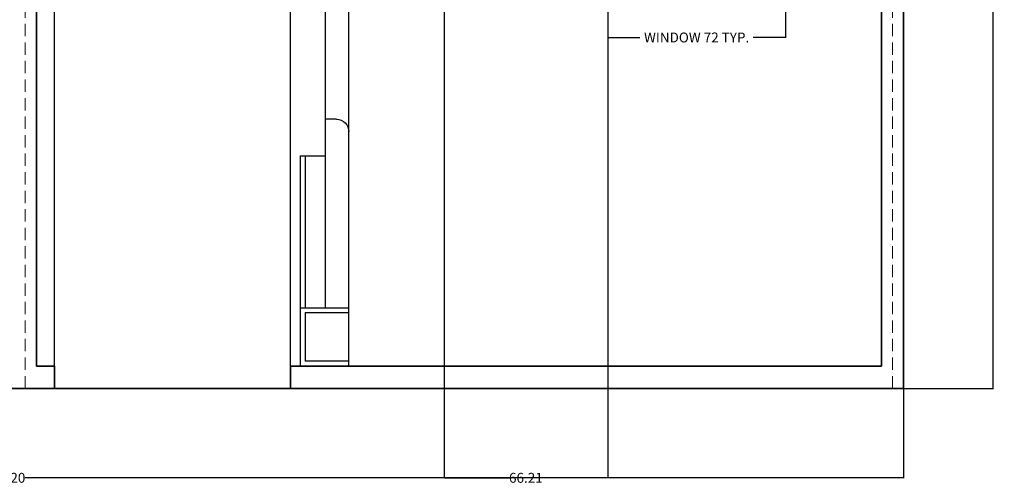
# Model space of a CAD drawing. Units: inches. Extents: x 1291 to 2095, y 532 to 1090.
# Tile 12 of 14: x 1696 to 2095, y 532 to 720. Entities that reach past the tile are written whole.
import ezdxf

# ---------------------------------------------------------------- set-up
doc = ezdxf.new("R2010")
doc.units = ezdxf.units.IN
doc.header["$MEASUREMENT"] = 0
doc.linetypes.add('HIDDEN', pattern=[0.375, 0.25, -0.125])
for name, color, linetype, lineweight in [('A-ANNO-DIMS', 2, 'Continuous', 18), ('A-WALL', 7, 'Continuous', 35), ('A-WALL-HIDN', 8, 'HIDDEN', 13), ('A-WALL-SITE', 7, 'Continuous', 25)]:
    doc.layers.add(name, color=color, linetype=linetype, lineweight=lineweight)
doc.styles.get("Standard").update_dxf_attribs({"font": 'arial.ttf'})
doc.dimstyles.get("Standard").update_dxf_attribs({"dimtxt": 4, "dimasz": 0.18, "dimexe": 0.18, "dimexo": 0.0625, "dimgap": 0.09, "dimtad": 0, "dimtih": 1, "dimtoh": 1, "dimdec": 0, "dimrnd": 6, "dimzin": 0, "dimdsep": 46, "dimlunit": 3, "dimtxsty": 'Standard', "dimcen": 0.09, "dimadec": 0, "dimazin": 0, "dimtfac": 1, "dimtdec": 0, "dimtofl": 0, "dimtmove": 0, "dimatfit": 3, "dimfxl": 1, "dimtolj": 1, "dimtzin": 0, "dimarcsym": 0})

# ---------------------------------------------------------------- blocks, each defined once
blk = doc.blocks.new('FRONT-COURT-DIVIDER')
for p, q in [((9.46, 23.64), (9.46, 144)), ((5, 99.92), (9.46, 99.92)), ((0, 0), (0, 94.92)), ((19.66, 85.14), (9.46, 85.14)), ((17.66, 85.14), (17.66, 23.64)), ((19.66, 85.14), (19.66, 0)), ((19.66, 23.64), (0, 23.64)), ((17.66, 21.64), (0, 21.64)), ((17.66, 21.64), (17.66, 2)), ((0, 2), (17.66, 2))]:
    blk.add_line(p, q)
blk.add_arc((5, 94.92), 5, 90, 180)
blk = doc.blocks.new('*D12')
at = {"layer": 'A-ANNO-DIMS', "color": 0, "lineweight": -2, "transparency": 16777216}
for p, q in [((1934.29, 723.52), (1934.29, 712.6)), ((2006.29, 723.52), (2006.29, 712.6)), ((1934.47, 712.78), (1947.34, 712.78)), ((2006.11, 712.78), (1993.23, 712.78))]:
    blk.add_line(p, q, dxfattribs=at)
at = {"layer": 'A-ANNO-DIMS', "color": 0, "transparency": 16777216}
for points in [[(1934.47, 712.81), (1934.47, 712.75), (1934.29, 712.78)], [(2006.11, 712.81), (2006.11, 712.75), (2006.29, 712.78)]]:
    blk.add_solid(points, dxfattribs=at)
at = {"layer": 'Defpoints', "color": 0, "transparency": 16777216}
for p in [(1934.29, 723.58), (2006.29, 723.58), (2006.29, 712.78)]:
    blk.add_point(p, dxfattribs=at)
at = {"layer": 'A-ANNO-DIMS', "color": 0, "transparency": 16777216, "insert": (1970.29, 712.78), "char_height": 4, "attachment_point": 5}
blk.add_mtext('\\A1;WINDOW 72 TYP.', dxfattribs=at)
blk = doc.blocks.new('*D32')
at = {"layer": 'A-ANNO-DIMS', "color": 0, "lineweight": -2, "transparency": 16777216}
for p, q in [((1334.07, 570.72), (1334.07, 534.4)), ((2054.07, 570.72), (2054.07, 534.4)), ((1334.25, 534.58), (1689.59, 534.58)), ((2053.89, 534.58), (1698.56, 534.58))]:
    blk.add_line(p, q, dxfattribs=at)
at = {"layer": 'A-ANNO-DIMS', "color": 0, "transparency": 16777216}
for points in [[(1334.25, 534.61), (1334.25, 534.55), (1334.07, 534.58)], [(2053.89, 534.61), (2053.89, 534.55), (2054.07, 534.58)]]:
    blk.add_solid(points, dxfattribs=at)
at = {"layer": 'Defpoints', "color": 0, "transparency": 16777216}
for p in [(1334.07, 570.78), (2054.07, 570.78), (2054.07, 534.58)]:
    blk.add_point(p, dxfattribs=at)
at = {"layer": 'A-ANNO-DIMS', "color": 0, "transparency": 16777216, "insert": (1694.07, 534.58), "char_height": 4, "attachment_point": 5}
blk.add_mtext('\\A1;720', dxfattribs=at)
blk = doc.blocks.new('*D33')
at = {"layer": 'A-ANNO-DIMS', "color": 0, "lineweight": -2, "transparency": 16777216}
for p, q in [((2054.14, 1050.78), (2090.45, 1050.78)), ((2090.27, 1050.6), (2090.27, 812.91)), ((2090.27, 570.96), (2090.27, 808.65)), ((2054.14, 570.78), (2090.45, 570.78))]:
    blk.add_line(p, q, dxfattribs=at)
at = {"layer": 'A-ANNO-DIMS', "color": 0, "transparency": 16777216}
for points in [[(2090.24, 1050.6), (2090.3, 1050.6), (2090.27, 1050.78)], [(2090.24, 570.96), (2090.3, 570.96), (2090.27, 570.78)]]:
    blk.add_solid(points, dxfattribs=at)
at = {"layer": 'Defpoints', "color": 0, "transparency": 16777216}
for p in [(2054.07, 1050.78), (2090.27, 1050.78), (2054.07, 570.78)]:
    blk.add_point(p, dxfattribs=at)
at = {"layer": 'A-ANNO-DIMS', "color": 0, "transparency": 16777216, "insert": (2090.27, 810.78), "char_height": 4, "attachment_point": 5}
blk.add_mtext('\\A1;480', dxfattribs=at)
blk = doc.blocks.new('*D45')
at = {"layer": 'A-ANNO-DIMS', "color": 0, "lineweight": -2, "transparency": 16777216}
for p, q in [((1829.54, 579.84), (1829.54, 1087.16)), ((1829.72, 1086.98), (1928.89, 1086.98)), ((2044.89, 1086.98), (1945.72, 1086.98)), ((2045.07, 579.84), (2045.07, 1087.16))]:
    blk.add_line(p, q, dxfattribs=at)
at = {"layer": 'A-ANNO-DIMS', "color": 0, "transparency": 16777216}
for points in [[(1829.72, 1087.01), (1829.72, 1086.95), (1829.54, 1086.98)], [(2044.89, 1087.01), (2044.89, 1086.95), (2045.07, 1086.98)]]:
    blk.add_solid(points, dxfattribs=at)
at = {"layer": 'Defpoints', "color": 0, "transparency": 16777216}
for p in [(2045.07, 1086.98), (1829.54, 579.78), (2045.07, 579.78)]:
    blk.add_point(p, dxfattribs=at)
at = {"layer": 'A-ANNO-DIMS', "color": 0, "transparency": 16777216, "insert": (1937.3, 1086.98), "char_height": 4, "attachment_point": 5}
blk.add_mtext('\\A1;215.54', dxfattribs=at)
blk = doc.blocks.new('*D47')
at = {"layer": 'A-ANNO-DIMS', "color": 0, "lineweight": -2, "transparency": 16777216}
for p, q in [((1710.36, 579.84), (1710.36, 1087.16)), ((1710.54, 1086.98), (1751.3, 1086.98)), ((1805.7, 1086.98), (1764.94, 1086.98)), ((1805.88, 579.84), (1805.88, 1087.16))]:
    blk.add_line(p, q, dxfattribs=at)
at = {"layer": 'A-ANNO-DIMS', "color": 0, "transparency": 16777216}
for points in [[(1710.54, 1087.01), (1710.54, 1086.95), (1710.36, 1086.98)], [(1805.7, 1087.01), (1805.7, 1086.95), (1805.88, 1086.98)]]:
    blk.add_solid(points, dxfattribs=at)
at = {"layer": 'Defpoints', "color": 0, "transparency": 16777216}
for p in [(1805.88, 1086.98), (1710.36, 579.78), (1805.88, 579.78)]:
    blk.add_point(p, dxfattribs=at)
at = {"layer": 'A-ANNO-DIMS', "color": 0, "transparency": 16777216, "insert": (1758.12, 1086.98), "char_height": 4, "attachment_point": 5}
blk.add_mtext('\\A1;95.52', dxfattribs=at)
blk = doc.blocks.new('*D68')
at = {"layer": 'A-ANNO-DIMS', "color": 0, "lineweight": -2, "transparency": 16777216}
for p, q in [((1868.07, 723.72), (1868.07, 534.4)), ((1934.29, 723.52), (1934.29, 534.4)), ((1868.25, 534.58), (1894.72, 534.58)), ((1934.11, 534.58), (1907.64, 534.58))]:
    blk.add_line(p, q, dxfattribs=at)
at = {"layer": 'A-ANNO-DIMS', "color": 0, "transparency": 16777216}
for points in [[(1868.25, 534.61), (1868.25, 534.55), (1868.07, 534.58)], [(1934.11, 534.61), (1934.11, 534.55), (1934.29, 534.58)]]:
    blk.add_solid(points, dxfattribs=at)
at = {"layer": 'Defpoints', "color": 0, "transparency": 16777216}
for p in [(1868.07, 723.78), (1934.29, 723.58), (1934.29, 534.58)]:
    blk.add_point(p, dxfattribs=at)
at = {"layer": 'A-ANNO-DIMS', "color": 0, "transparency": 16777216, "insert": (1901.18, 534.58), "char_height": 4, "attachment_point": 5}
blk.add_mtext('\\A1;66.21', dxfattribs=at)

msp = doc.modelspace()

# ---------------------------------------------------------------- linework, layer by layer
at = {"layer": 'A-WALL'}
for p, q in [((2054.0735, 570.7804), (2054.0735, 1050.7804)), ((1703.0735, 579.7804), (1703.0735, 723.7804)), ((2045.0735, 579.7804), (2045.0735, 723.7804)), ((1703.0735, 579.7804), (1710.3593, 579.7804)), ((1710.3593, 579.7804), (1710.3593, 570.7804)), ((1805.8774, 579.7804), (2045.0735, 579.7804)), ((1805.8774, 579.7804), (1805.8774, 570.7804)), ((1685.5842, 570.7804), (1710.3593, 570.7804)), ((1710.3593, 570.7804), (2054.0735, 570.7804))]:
    msp.add_line(p, q, dxfattribs=at)
at = {"layer": 'A-WALL-HIDN', "ltscale": 20}
for p, q in [((1698.5735, 570.7804), (1698.5735, 1046.2804)), ((2049.5735, 570.7804), (2049.5735, 1046.2804))]:
    msp.add_line(p, q, dxfattribs=at)
at = {"layer": 'A-WALL-SITE'}
msp.add_line((1820.0735, 603.4219), (1820.0735, 679.6964), dxfattribs=at)

# ---------------------------------------------------------------- block references
at = {"layer": 'A-WALL-SITE', "extrusion": (0, 0, -1), "zscale": -1}
msp.add_blockref('FRONT-COURT-DIVIDER', (-1829.5361, 579.78), dxfattribs=at)

# ---------------------------------------------------------------- dimensions: what is measured, and where the dimension line sits
at = {"layer": 'A-ANNO-DIMS'}
for base, p1, p2, override, picture, middle in [((1805.8774, 1086.9804), (1710.3593, 579.7804), (1805.8774, 579.7804), {"dimdec": 2, "dimlfac": 1, "dimrnd": 0, "dimzin": 0, "dimdsep": 46, "dimlunit": 2}, '*D47', (1758.1183, 1086.9804)), ((2045.0735, 1086.9804), (1829.5364, 579.7804), (2045.0735, 579.7804), {"dimdec": 2, "dimlfac": 1, "dimrnd": 0, "dimzin": 0, "dimdsep": 46, "dimlunit": 2}, '*D45', (1937.3049, 1086.9804)), ((1934.2856, 534.5804), (1868.0735, 723.7804), (1934.2856, 723.5846), {"dimdec": 2, "dimlfac": 1, "dimrnd": 0, "dimzin": 0, "dimdsep": 46, "dimlunit": 2}, '*D68', (1901.1796, 534.5804)), ((2054.0735, 534.5804), (1334.0735, 570.7804), (2054.0735, 570.7804), {"dimdec": 0, "dimlfac": 1, "dimrnd": 0, "dimzin": 0, "dimdsep": 46, "dimlunit": 2}, '*D32', (1694.0735, 534.5804))]:
    dim = msp.add_linear_dim(base=base, p1=p1, p2=p2, dimstyle='Standard', override=override, dxfattribs=at)
    dim.commit()
    dim.dimension.update_dxf_attribs({"geometry": picture, "text_midpoint": middle})
dim = msp.add_linear_dim(base=(2090.2735, 1050.7804), p1=(2054.0735, 570.7804), p2=(2054.0735, 1050.7804), angle=90, dimstyle='Standard', override={"dimdec": 0, "dimlfac": 1, "dimrnd": 0, "dimzin": 0, "dimdsep": 46, "dimlunit": 2}, dxfattribs=at)
dim.commit()
dim.dimension.update_dxf_attribs({"geometry": '*D33', "text_midpoint": (2090.2735, 810.7804)})
dim = msp.add_linear_dim(base=(2006.2856, 712.7846), p1=(1934.2856, 723.5846), p2=(2006.2856, 723.5846), text='WINDOW <> TYP.', dimstyle='Standard', override={"dimdec": 0, "dimlfac": 1, "dimrnd": 0, "dimzin": 0, "dimdsep": 46, "dimlunit": 2}, dxfattribs=at)
dim.commit()
dim.dimension.update_dxf_attribs({"geometry": '*D12', "text_midpoint": (1970.2856, 712.7846)})

doc.saveas('drawing.dxf')
